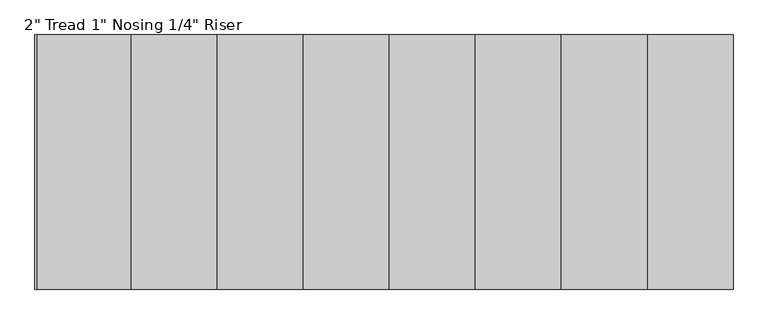
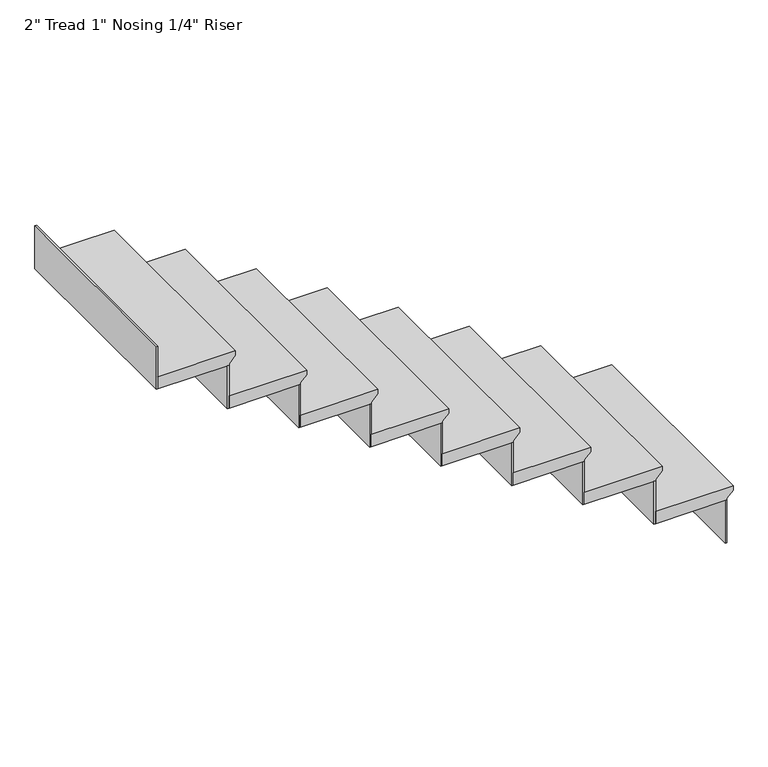
"""IFC4 building model written with IfcOpenShell, lengths in millimetres: stair flight geometry."""

from ifc_helpers import new_model, si_unit, frame, origin, place, context, project, spatial, polyline, outline, extrude, source, transform, mapped, element, save


def stair_flight_c84ce1c3(model_context):
    return source(origin(), model_context, "Body", "SweptSolid", [
        extrude(outline(polyline([(1778.0, -2950.6837185), (1778.0, -3255.4837185), (1727.2, -3255.4837185), (1727.2, -2976.0837185), (1733.55, -2976.0837185), (1758.95, -2950.6837185), (1778.0, -2950.6837185)])), frame((0.0, -8000.7366292, 0.0), z_axis=(0.0, 1.0, 0.0), x_axis=(0.0, 0.0, 1.0)), (0.0, 0.0, 1.0), 826.6488507),
        extrude(outline(polyline([(-2982.4337185, -7174.0877785), (-2976.0837185, -7174.0877785), (-2976.0837185, -8000.7366292), (-2982.4337185, -8000.7366292), (-2982.4337185, -7174.0877785)])), frame((0.0, 0.0, 1549.4), z_axis=(0.0, 0.0, 1.0), x_axis=(1.0, 0.0, 0.0)), (0.0, 0.0, 1.0), 177.8),
        extrude(outline(polyline([(-3261.8337185, -7174.0877785), (-3255.4837185, -7174.0877785), (-3255.4837185, -8000.7366292), (-3261.8337185, -8000.7366292), (-3261.8337185, -7174.0877785)])), frame((0.0, 0.0, 1727.2), z_axis=(0.0, 0.0, 1.0), x_axis=(1.0, 0.0, 0.0)), (0.0, 0.0, 1.0), 177.8),
        extrude(outline(polyline([(1955.8, -3230.0837185), (1955.8, -3534.8837185), (1905.0, -3534.8837185), (1905.0, -3255.4837185), (1911.35, -3255.4837185), (1936.75, -3230.0837185), (1955.8, -3230.0837185)])), frame((0.0, -8000.7366292, 0.0), z_axis=(0.0, 1.0, 0.0), x_axis=(0.0, 0.0, 1.0)), (0.0, 0.0, 1.0), 826.6488507),
        extrude(outline(polyline([(-3541.2337185, -7174.0877785), (-3534.8837185, -7174.0877785), (-3534.8837185, -8000.7366292), (-3541.2337185, -8000.7366292), (-3541.2337185, -7174.0877785)])), frame((0.0, 0.0, 1905.0), z_axis=(0.0, 0.0, 1.0), x_axis=(1.0, 0.0, 0.0)), (0.0, 0.0, 1.0), 177.8),
        extrude(outline(polyline([(2133.6, -3509.4837185), (2133.6, -3814.2837185), (2082.8, -3814.2837185), (2082.8, -3534.8837185), (2089.15, -3534.8837185), (2114.55, -3509.4837185), (2133.6, -3509.4837185)])), frame((0.0, -8000.7366292, 0.0), z_axis=(0.0, 1.0, 0.0), x_axis=(0.0, 0.0, 1.0)), (0.0, 0.0, 1.0), 826.6488507),
        extrude(outline(polyline([(-3820.6337185, -7174.0877785), (-3814.2837185, -7174.0877785), (-3814.2837185, -8000.7366292), (-3820.6337185, -8000.7366292), (-3820.6337185, -7174.0877785)])), frame((0.0, 0.0, 2082.8), z_axis=(0.0, 0.0, 1.0), x_axis=(1.0, 0.0, 0.0)), (0.0, 0.0, 1.0), 177.8),
        extrude(outline(polyline([(2311.4, -3788.8837185), (2311.4, -4093.6837185), (2260.6, -4093.6837185), (2260.6, -3814.2837185), (2266.95, -3814.2837185), (2292.35, -3788.8837185), (2311.4, -3788.8837185)])), frame((0.0, -8000.7366292, 0.0), z_axis=(0.0, 1.0, 0.0), x_axis=(0.0, 0.0, 1.0)), (0.0, 0.0, 1.0), 826.6488507),
        extrude(outline(polyline([(-4100.0337185, -7174.0877785), (-4093.6837185, -7174.0877785), (-4093.6837185, -8000.7366292), (-4100.0337185, -8000.7366292), (-4100.0337185, -7174.0877785)])), frame((0.0, 0.0, 2260.6), z_axis=(0.0, 0.0, 1.0), x_axis=(1.0, 0.0, 0.0)), (0.0, 0.0, 1.0), 177.8),
        extrude(outline(polyline([(2489.2, -4068.2837185), (2489.2, -4373.0837185), (2438.4, -4373.0837185), (2438.4, -4093.6837185), (2444.75, -4093.6837185), (2470.15, -4068.2837185), (2489.2, -4068.2837185)])), frame((0.0, -8000.7366292, 0.0), z_axis=(0.0, 1.0, 0.0), x_axis=(0.0, 0.0, 1.0)), (0.0, 0.0, 1.0), 826.6488507),
        extrude(outline(polyline([(-4379.4337185, -7174.0877785), (-4373.0837185, -7174.0877785), (-4373.0837185, -8000.7366292), (-4379.4337185, -8000.7366292), (-4379.4337185, -7174.0877785)])), frame((0.0, 0.0, 2438.4), z_axis=(0.0, 0.0, 1.0), x_axis=(1.0, 0.0, 0.0)), (0.0, 0.0, 1.0), 177.8),
        extrude(outline(polyline([(2667.0, -4347.6837185), (2667.0, -4652.4837185), (2616.2, -4652.4837185), (2616.2, -4373.0837185), (2622.55, -4373.0837185), (2647.95, -4347.6837185), (2667.0, -4347.6837185)])), frame((0.0, -8000.7366292, 0.0), z_axis=(0.0, 1.0, 0.0), x_axis=(0.0, 0.0, 1.0)), (0.0, 0.0, 1.0), 826.6488507),
        extrude(outline(polyline([(-4658.8337185, -7174.0877785), (-4652.4837185, -7174.0877785), (-4652.4837185, -8000.7366292), (-4658.8337185, -8000.7366292), (-4658.8337185, -7174.0877785)])), frame((0.0, 0.0, 2616.2), z_axis=(0.0, 0.0, 1.0), x_axis=(1.0, 0.0, 0.0)), (0.0, 0.0, 1.0), 177.8),
        extrude(outline(polyline([(2844.8, -4627.0837185), (2844.8, -4931.8837185), (2794.0, -4931.8837185), (2794.0, -4652.4837185), (2800.35, -4652.4837185), (2825.75, -4627.0837185), (2844.8, -4627.0837185)])), frame((0.0, -8000.7366292, 0.0), z_axis=(0.0, 1.0, 0.0), x_axis=(0.0, 0.0, 1.0)), (0.0, 0.0, 1.0), 826.6488507),
        extrude(outline(polyline([(-4938.2337185, -7174.0877785), (-4931.8837185, -7174.0877785), (-4931.8837185, -8000.7366292), (-4938.2337185, -8000.7366292), (-4938.2337185, -7174.0877785)])), frame((0.0, 0.0, 2794.0), z_axis=(0.0, 0.0, 1.0), x_axis=(1.0, 0.0, 0.0)), (0.0, 0.0, 1.0), 177.8),
        extrude(outline(polyline([(-5217.6337185, -7174.0877785), (-5211.2837185, -7174.0877785), (-5211.2837185, -8000.7366292), (-5217.6337185, -8000.7366292), (-5217.6337185, -7174.0877785)])), frame((0.0, 0.0, 2971.8), z_axis=(0.0, 0.0, 1.0), x_axis=(1.0, 0.0, 0.0)), (0.0, 0.0, 1.0), 177.8),
        extrude(outline(polyline([(3022.6, -4906.4837185), (3022.6, -5211.2837185), (2971.8, -5211.2837185), (2971.8, -4931.8837185), (2978.15, -4931.8837185), (3003.55, -4906.4837185), (3022.6, -4906.4837185)])), frame((0.0, -8000.7366292, 0.0), z_axis=(0.0, 1.0, 0.0), x_axis=(0.0, 0.0, 1.0)), (0.0, 0.0, 1.0), 826.6488507),
    ])


if __name__ == "__main__":
    model = new_model("IFC4")
    model_context = context("Model", 3, world=origin())
    ifc_project = project(units=[si_unit("LENGTHUNIT", "METRE", prefix="MILLI")], contexts=[model_context])
    site = spatial("IfcSite", under=ifc_project)
    building = spatial("IfcBuilding", under=site)
    placement = place(None, origin())
    stair_flight_shape = stair_flight_c84ce1c3(model_context)
    element("IfcStairFlight", 1, ObjectType="2\" Tread 1\" Nosing 1/4\" Riser", at=placement, inside=building, context=model_context, shape_type="MappedRepresentation", body=[
        mapped(stair_flight_shape, transform((0.0, 0.0, 0.0), x_axis=(1.0, 0.0, 0.0), y_axis=(0.0, 1.0, 0.0), z_axis=(0.0, 0.0, 1.0))),
    ])
    save(model, "model.ifc")
